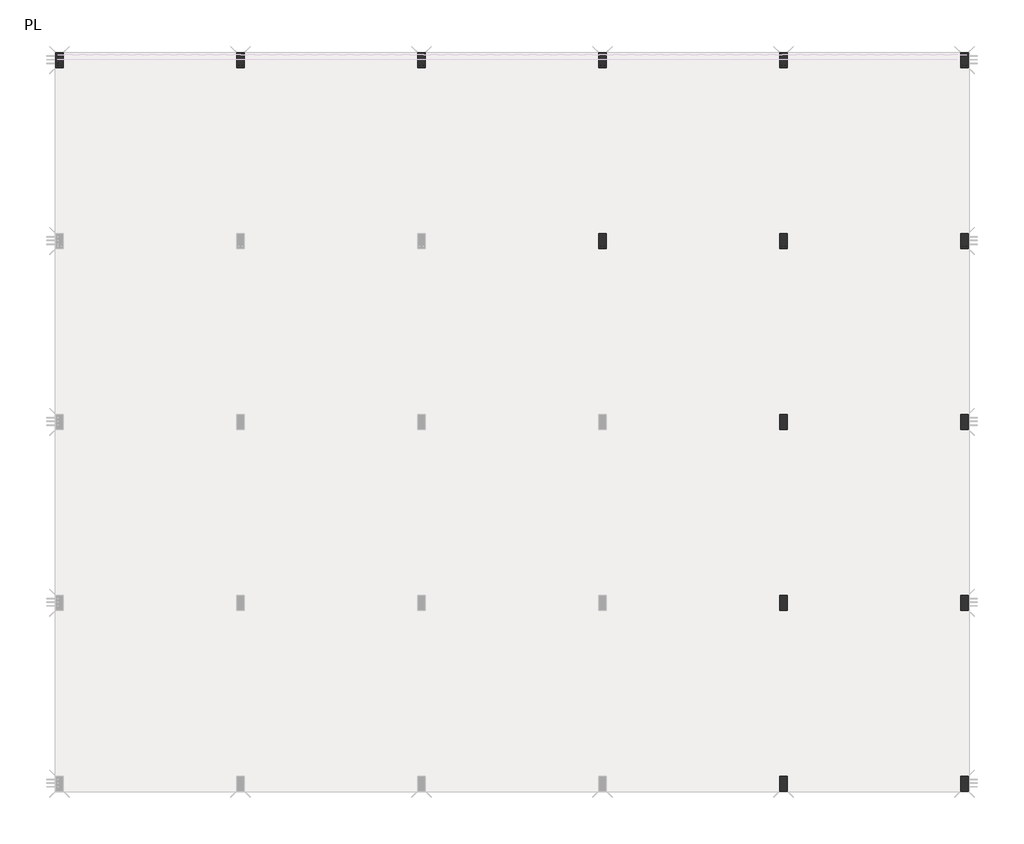
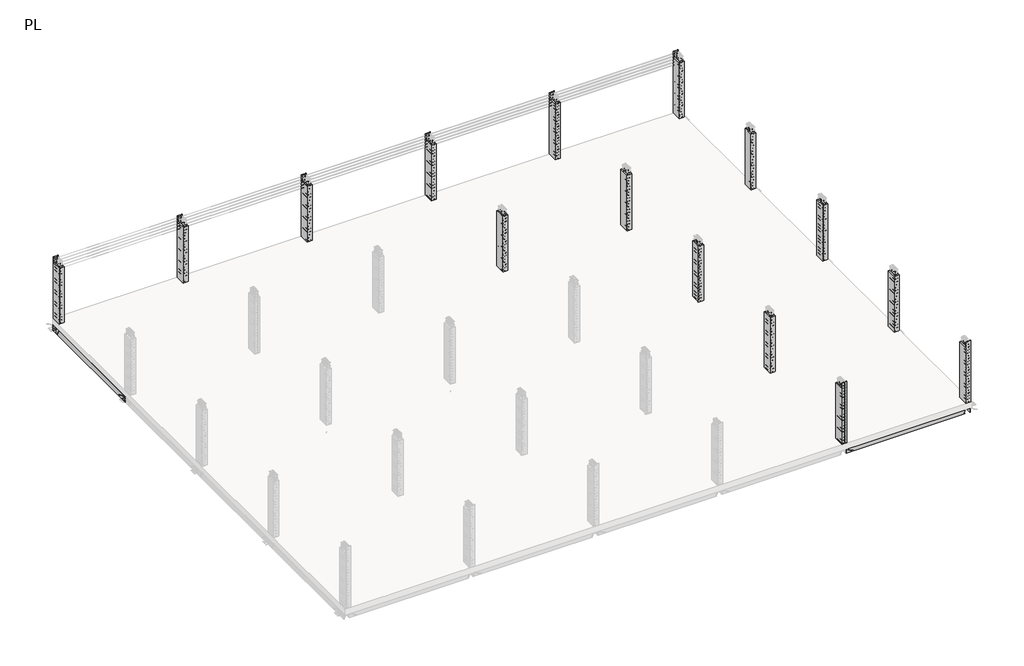
# One storey, part 2 of 10: 25 beams, 15 columns.
"""IFC4 building model written with IfcOpenShell, lengths in millimetres."""

from ifc_helpers import new_model, si_unit, frame, origin, place, context, project, spatial, polyline, outline, extrude, faceted_brep, element, save

model = new_model("IFC4")

# Units and contexts
model_context = context("Model", 3, world=origin())
ifc_project = project(units=[si_unit("LENGTHUNIT", "METRE", prefix="MILLI")], contexts=[model_context])

# Site, building, storey
site = spatial("IfcSite", under=ifc_project)
building = spatial("IfcBuilding", under=site)
storey = spatial("IfcBuildingStorey", under=building, Name="PL", Elevation=271.0)

# Beams
placement = place(None, origin())
element("IfcBeam", 1, ObjectType="Concrete-Rectangular Beam : 300 x 600mm", at=placement, inside=storey, context=model_context, shape_type="Brep", body=[
    faceted_brep([(7798.0455621, 4054.0653602, -329.0), (7823.0455621, 4054.0653602, -329.0), (7823.0455621, 4054.0653602, -29.0), (7798.0455621, 4054.0653602, -29.0), (7823.0455621, 4354.0653602, -329.0), (7798.0455621, 4354.0653602, -329.0), (7798.0455621, 4354.0653602, -29.0), (7823.0455621, 4354.0653602, -29.0)], [[[0, 1, 2, 3]], [[4, 1, 0, 5]], [[4, 5, 6, 7]], [[1, 4, 7, 2]], [[5, 0, 3, 6]], [[3, 2, 7, 6]]]),
    faceted_brep([(-22681.9544379, 4354.0653602, -329.0), (-22681.9544379, 4054.0653602, -329.0), (-22681.9544379, 4054.0653602, -29.0), (-22681.9544379, 4354.0653602, -29.0), (-16835.9544379, 4054.0653602, -329.0), (-16835.9544379, 4354.0653602, -329.0), (-16835.9544379, 4354.0653602, -29.0), (-16835.9544379, 4054.0653602, -29.0), (-22656.9544379, 4054.0653602, -329.0), (-16860.9544379, 4054.0653602, -329.0), (-16860.9544379, 4054.0653602, -29.0), (-22656.9544379, 4054.0653602, -29.0)], [[[0, 1, 2, 3]], [[4, 5, 6, 7]], [[1, 8, 9, 4, 7, 10, 11, 2]], [[1, 0, 5, 4, 9, 8]], [[5, 0, 3, 6]], [[3, 2, 11, 10, 7, 6]]]),
    faceted_brep([(7548.0455621, 4054.0653602, -329.0), (7548.0455621, 4354.0653602, -329.0), (7548.0455621, 4354.0653602, -29.0), (7548.0455621, 4054.0653602, -29.0), (1702.0455621, 4354.0653602, -329.0), (1702.0455621, 4054.0653602, -329.0), (1702.0455621, 4054.0653602, -29.0), (1702.0455621, 4354.0653602, -29.0), (1727.0455621, 4054.0653602, -329.0), (7523.0455621, 4054.0653602, -329.0), (7523.0455621, 4054.0653602, -29.0), (1727.0455621, 4054.0653602, -29.0)], [[[0, 1, 2, 3]], [[4, 5, 6, 7]], [[5, 8, 9, 0, 3, 10, 11, 6]], [[1, 0, 9, 8, 5, 4]], [[1, 4, 7, 2]], [[3, 2, 7, 6, 11, 10]]]),
    faceted_brep([(-16585.9544379, 4354.0653602, -329.0), (-16585.9544379, 4054.0653602, -329.0), (-16585.9544379, 4054.0653602, -29.0), (-16585.9544379, 4354.0653602, -29.0), (-10739.9544379, 4054.0653602, -329.0), (-10739.9544379, 4354.0653602, -329.0), (-10739.9544379, 4354.0653602, -29.0), (-10739.9544379, 4054.0653602, -29.0)], [[[0, 1, 2, 3]], [[4, 5, 6, 7]], [[1, 4, 7, 2]], [[1, 0, 5, 4]], [[5, 0, 3, 6]], [[3, 2, 7, 6]]]),
    faceted_brep([(-10489.9544379, 4354.0653602, -329.0), (-10489.9544379, 4054.0653602, -329.0), (-10489.9544379, 4054.0653602, -29.0), (-10489.9544379, 4354.0653602, -29.0), (-4643.9544379, 4054.0653602, -329.0), (-4643.9544379, 4354.0653602, -329.0), (-4643.9544379, 4354.0653602, -29.0), (-4643.9544379, 4054.0653602, -29.0), (-10464.9544379, 4054.0653602, -329.0), (-10464.9544379, 4054.0653602, -29.0)], [[[0, 1, 2, 3]], [[4, 5, 6, 7]], [[1, 8, 4, 7, 9, 2]], [[1, 0, 5, 4, 8]], [[5, 0, 3, 6]], [[3, 2, 9, 7, 6]]]),
    faceted_brep([(-4393.9544379, 4354.0653602, -329.0), (-4393.9544379, 4054.0653602, -329.0), (-4393.9544379, 4054.0653602, -29.0), (-4393.9544379, 4354.0653602, -29.0), (1452.0455621, 4054.0653602, -329.0), (1452.0455621, 4354.0653602, -329.0), (1452.0455621, 4354.0653602, -29.0), (1452.0455621, 4054.0653602, -29.0), (-4368.9544379, 4054.0653602, -329.0), (-4368.9544379, 4054.0653602, -29.0)], [[[0, 1, 2, 3]], [[4, 5, 6, 7]], [[1, 8, 4, 7, 9, 2]], [[1, 0, 5, 4, 8]], [[5, 0, 3, 6]], [[3, 2, 9, 7, 6]]]),
    faceted_brep([(-22956.9544379, 4354.0653602, -329.0), (-22956.9544379, 4054.0653602, -329.0), (-22956.9544379, 4054.0653602, -29.0), (-22956.9544379, 4354.0653602, -29.0), (-22931.9544379, 4054.0653602, -329.0), (-22931.9544379, 4354.0653602, -329.0), (-22931.9544379, 4354.0653602, -29.0), (-22931.9544379, 4054.0653602, -29.0)], [[[0, 1, 2, 3]], [[4, 5, 6, 7]], [[1, 4, 7, 2]], [[1, 0, 5, 4]], [[5, 0, 3, 6]], [[3, 2, 7, 6]]]),
])
element("IfcBeam", 2, ObjectType="Concrete-Rectangular Beam : 300 x 600mm", at=placement, inside=storey, context=model_context, shape_type="Brep", body=[
    faceted_brep([(7798.0455621, -20429.1167521, -329.0), (7823.0455621, -20429.1167521, -329.0), (7823.0455621, -20429.1167521, -29.0), (7798.0455621, -20429.1167521, -29.0), (7823.0455621, -20129.1167521, -329.0), (7798.0455621, -20129.1167521, -329.0), (7798.0455621, -20129.1167521, -29.0), (7823.0455621, -20129.1167521, -29.0)], [[[0, 1, 2, 3]], [[4, 1, 0, 5]], [[4, 5, 6, 7]], [[1, 4, 7, 2]], [[5, 0, 3, 6]], [[3, 2, 7, 6]]]),
    faceted_brep([(1727.0455621, -20129.1167521, -329.0), (1727.0455621, -20429.1167521, -329.0), (1727.0455621, -20429.1167521, -29.0), (1727.0455621, -20129.1167521, -29.0), (7548.0455621, -20429.1167521, -329.0), (7548.0455621, -20129.1167521, -329.0), (7548.0455621, -20129.1167521, -29.0), (7548.0455621, -20429.1167521, -29.0), (7523.0455621, -20129.1167521, -329.0), (7523.0455621, -20129.1167521, -29.0)], [[[0, 1, 2, 3]], [[4, 5, 6, 7]], [[1, 4, 7, 2]], [[1, 0, 8, 5, 4]], [[5, 8, 0, 3, 9, 6]], [[3, 2, 7, 6, 9]]]),
])
element("IfcBeam", 3, ObjectType="Concrete-Rectangular Beam : 300 x 600mm", at=placement, inside=storey, context=model_context, shape_type="Brep", body=[
    faceted_brep([(7798.0455621, -14333.1167521, -329.0), (7823.0455621, -14333.1167521, -329.0), (7823.0455621, -14333.1167521, -29.0), (7798.0455621, -14333.1167521, -29.0), (7823.0455621, -14033.1167521, -329.0), (7798.0455621, -14033.1167521, -329.0), (7798.0455621, -14033.1167521, -29.0), (7823.0455621, -14033.1167521, -29.0)], [[[0, 1, 2, 3]], [[4, 1, 0, 5]], [[4, 5, 6, 7]], [[1, 4, 7, 2]], [[5, 0, 3, 6]], [[3, 2, 7, 6]]]),
    faceted_brep([(1727.0455621, -14033.1167521, -329.0), (1727.0455621, -14333.1167521, -329.0), (1727.0455621, -14333.1167521, -29.0), (1727.0455621, -14033.1167521, -29.0), (7548.0455621, -14333.1167521, -329.0), (7548.0455621, -14033.1167521, -329.0), (7548.0455621, -14033.1167521, -29.0), (7548.0455621, -14333.1167521, -29.0), (7523.0455621, -14333.1167521, -329.0), (7523.0455621, -14333.1167521, -29.0), (7523.0455621, -14033.1167521, -329.0), (7523.0455621, -14033.1167521, -29.0)], [[[0, 1, 2, 3]], [[4, 5, 6, 7]], [[1, 8, 4, 7, 9, 2]], [[1, 0, 10, 5, 4, 8]], [[5, 10, 0, 3, 11, 6]], [[3, 2, 9, 7, 6, 11]]]),
])
element("IfcBeam", 4, ObjectType="Concrete-Rectangular Beam : 300 x 600mm", at=placement, inside=storey, context=model_context, shape_type="Brep", body=[
    faceted_brep([(7798.0455621, -8237.1167521, -329.0), (7823.0455621, -8237.1167521, -329.0), (7823.0455621, -8237.1167521, -29.0), (7798.0455621, -8237.1167521, -29.0), (7823.0455621, -7937.1167521, -329.0), (7798.0455621, -7937.1167521, -329.0), (7798.0455621, -7937.1167521, -29.0), (7823.0455621, -7937.1167521, -29.0)], [[[0, 1, 2, 3]], [[4, 1, 0, 5]], [[4, 5, 6, 7]], [[1, 4, 7, 2]], [[5, 0, 3, 6]], [[3, 2, 7, 6]]]),
    faceted_brep([(1727.0455621, -7937.1167521, -329.0), (1727.0455621, -8237.1167521, -329.0), (1727.0455621, -8237.1167521, -29.0), (1727.0455621, -7937.1167521, -29.0), (7548.0455621, -8237.1167521, -329.0), (7548.0455621, -7937.1167521, -329.0), (7548.0455621, -7937.1167521, -29.0), (7548.0455621, -8237.1167521, -29.0), (7523.0455621, -8237.1167521, -329.0), (7523.0455621, -8237.1167521, -29.0), (7523.0455621, -7937.1167521, -329.0), (7523.0455621, -7937.1167521, -29.0)], [[[0, 1, 2, 3]], [[4, 5, 6, 7]], [[1, 8, 4, 7, 9, 2]], [[1, 0, 10, 5, 4, 8]], [[5, 10, 0, 3, 11, 6]], [[3, 2, 9, 7, 6, 11]]]),
])
element("IfcBeam", 5, ObjectType="Concrete-Rectangular Beam : 300 x 600mm", at=placement, inside=storey, context=model_context, shape_type="Brep", body=[
    faceted_brep([(-4393.9544379, -2141.1167521, -329.0), (-4368.9544379, -2141.1167521, -329.0), (-4368.9544379, -2141.1167521, -29.0), (-4393.9544379, -2141.1167521, -29.0), (-4368.9544379, -1841.1167521, -329.0), (-4393.9544379, -1841.1167521, -329.0), (-4393.9544379, -1841.1167521, -29.0), (-4368.9544379, -1841.1167521, -29.0)], [[[0, 1, 2, 3]], [[4, 1, 0, 5]], [[4, 5, 6, 7]], [[1, 4, 7, 2]], [[5, 0, 3, 6]], [[3, 2, 7, 6]]]),
    faceted_brep([(-10464.9544379, -1841.1167521, -329.0), (-10464.9544379, -2141.1167521, -329.0), (-10464.9544379, -2141.1167521, -29.0), (-10464.9544379, -1841.1167521, -29.0), (-4643.9544379, -2141.1167521, -329.0), (-4643.9544379, -1841.1167521, -329.0), (-4643.9544379, -1841.1167521, -29.0), (-4643.9544379, -2141.1167521, -29.0), (-4668.9544379, -2141.1167521, -329.0), (-4668.9544379, -2141.1167521, -29.0), (-4668.9544379, -1841.1167521, -329.0), (-4668.9544379, -1841.1167521, -29.0)], [[[0, 1, 2, 3]], [[4, 5, 6, 7]], [[1, 8, 4, 7, 9, 2]], [[1, 0, 10, 5, 4, 8]], [[5, 10, 0, 3, 11, 6]], [[3, 2, 9, 7, 6, 11]]]),
])
element("IfcBeam", 6, ObjectType="Concrete-Rectangular Beam : 300 x 600mm", at=placement, inside=storey, context=model_context, shape_type="Brep", body=[
    faceted_brep([(1702.0455621, -2141.1167521, -329.0), (1727.0455621, -2141.1167521, -329.0), (1727.0455621, -2141.1167521, -29.0), (1702.0455621, -2141.1167521, -29.0), (1727.0455621, -1841.1167521, -329.0), (1702.0455621, -1841.1167521, -329.0), (1702.0455621, -1841.1167521, -29.0), (1727.0455621, -1841.1167521, -29.0)], [[[0, 1, 2, 3]], [[4, 1, 0, 5]], [[4, 5, 6, 7]], [[1, 4, 7, 2]], [[5, 0, 3, 6]], [[3, 2, 7, 6]]]),
    faceted_brep([(-4368.9544379, -1841.1167521, -329.0), (-4368.9544379, -2141.1167521, -329.0), (-4368.9544379, -2141.1167521, -29.0), (-4368.9544379, -1841.1167521, -29.0), (1452.0455621, -2141.1167521, -329.0), (1452.0455621, -1841.1167521, -329.0), (1452.0455621, -1841.1167521, -29.0), (1452.0455621, -2141.1167521, -29.0), (1427.0455621, -2141.1167521, -329.0), (1427.0455621, -2141.1167521, -29.0), (1427.0455621, -1841.1167521, -329.0), (1427.0455621, -1841.1167521, -29.0)], [[[0, 1, 2, 3]], [[4, 5, 6, 7]], [[1, 8, 4, 7, 9, 2]], [[1, 0, 10, 5, 4, 8]], [[5, 10, 0, 3, 11, 6]], [[3, 2, 9, 7, 6, 11]]]),
])
element("IfcBeam", 7, ObjectType="Concrete-Rectangular Beam : 300 x 600mm", at=placement, inside=storey, context=model_context, shape_type="Brep", body=[
    faceted_brep([(7798.0455621, -2141.1167521, -329.0), (7823.0455621, -2141.1167521, -329.0), (7823.0455621, -2141.1167521, -29.0), (7798.0455621, -2141.1167521, -29.0), (7823.0455621, -1841.1167521, -329.0), (7798.0455621, -1841.1167521, -329.0), (7798.0455621, -1841.1167521, -29.0), (7823.0455621, -1841.1167521, -29.0)], [[[0, 1, 2, 3]], [[4, 1, 0, 5]], [[4, 5, 6, 7]], [[1, 4, 7, 2]], [[5, 0, 3, 6]], [[3, 2, 7, 6]]]),
    faceted_brep([(1727.0455621, -1841.1167521, -329.0), (1727.0455621, -2141.1167521, -329.0), (1727.0455621, -2141.1167521, -29.0), (1727.0455621, -1841.1167521, -29.0), (7548.0455621, -2141.1167521, -329.0), (7548.0455621, -1841.1167521, -329.0), (7548.0455621, -1841.1167521, -29.0), (7548.0455621, -2141.1167521, -29.0), (7523.0455621, -2141.1167521, -329.0), (7523.0455621, -2141.1167521, -29.0), (7523.0455621, -1841.1167521, -329.0), (7523.0455621, -1841.1167521, -29.0)], [[[0, 1, 2, 3]], [[4, 5, 6, 7]], [[1, 8, 4, 7, 9, 2]], [[1, 0, 10, 5, 4, 8]], [[5, 10, 0, 3, 11, 6]], [[3, 2, 9, 7, 6, 11]]]),
])
element("IfcBeam", 8, ObjectType="Concrete-Rectangular Beam : 300 x 600mm", at=placement, inside=storey, context=model_context, shape_type="Brep", body=[
    faceted_brep([(-10489.9544379, 3954.8832479, -329.0), (-10464.9544379, 3954.8832479, -329.0), (-10464.9544379, 3954.8832479, -29.0), (-10489.9544379, 3954.8832479, -29.0), (-10464.9544379, 4054.0653602, -329.0), (-10489.9544379, 4054.0653602, -329.0), (-10464.9544379, 4054.0653602, -29.0), (-10489.9544379, 4054.0653602, -29.0)], [[[0, 1, 2, 3]], [[4, 1, 0, 5]], [[1, 4, 6, 2]], [[5, 0, 3, 7]], [[4, 5, 7, 6]], [[3, 2, 6, 7]]]),
    faceted_brep([(-16860.9544379, 4054.0653602, -329.0), (-16860.9544379, 3954.8832479, -329.0), (-16860.9544379, 3954.8832479, -29.0), (-16860.9544379, 4054.0653602, -29.0), (-16835.9544379, 3954.8832479, -329.0), (-16835.9544379, 4054.0653602, -329.0), (-16835.9544379, 4054.0653602, -29.0), (-16835.9544379, 3954.8832479, -29.0)], [[[0, 1, 2, 3]], [[4, 5, 6, 7]], [[1, 4, 7, 2]], [[1, 0, 5, 4]], [[5, 0, 3, 6]], [[3, 2, 7, 6]]]),
    faceted_brep([(-10739.9544379, 3954.8832479, -329.0), (-10739.9544379, 4054.0653602, -329.0), (-10739.9544379, 4054.0653602, -29.0), (-10739.9544379, 3954.8832479, -29.0), (-16585.9544379, 3954.8832479, -329.0), (-16560.9544379, 3954.8832479, -329.0), (-10764.9544379, 3954.8832479, -329.0), (-10764.9544379, 3954.8832479, -29.0), (-16560.9544379, 3954.8832479, -29.0), (-16585.9544379, 3954.8832479, -29.0), (-16585.9544379, 4054.0653602, -329.0), (-16585.9544379, 4054.0653602, -29.0)], [[[0, 1, 2, 3]], [[4, 5, 6, 0, 3, 7, 8, 9]], [[1, 0, 6, 5, 4, 10]], [[1, 10, 11, 2]], [[10, 4, 9, 11]], [[3, 2, 11, 9, 8, 7]]]),
])
element("IfcBeam", 9, ObjectType="Concrete-Rectangular Beam : 300 x 600mm", at=placement, inside=storey, context=model_context, shape_type="Brep", body=[
    faceted_brep([(-4393.9544379, 3954.8832479, -329.0), (-4368.9544379, 3954.8832479, -329.0), (-4368.9544379, 3954.8832479, -29.0), (-4393.9544379, 3954.8832479, -29.0), (-4393.9544379, 4054.0653602, -329.0), (-4368.9544379, 4054.0653602, -329.0), (-4368.9544379, 4054.0653602, -29.0), (-4393.9544379, 4054.0653602, -29.0)], [[[0, 1, 2, 3]], [[1, 0, 4, 5]], [[1, 5, 6, 2]], [[4, 0, 3, 7]], [[5, 4, 7, 6]], [[3, 2, 6, 7]]]),
    faceted_brep([(-10464.9544379, 4054.0653602, -329.0), (-10464.9544379, 3954.8832479, -329.0), (-10464.9544379, 3954.8832479, -29.0), (-10464.9544379, 4054.0653602, -29.0), (-4643.9544379, 3954.8832479, -329.0), (-4643.9544379, 4054.0653602, -329.0), (-4643.9544379, 4054.0653602, -29.0), (-4643.9544379, 3954.8832479, -29.0), (-4668.9544379, 3954.8832479, -329.0), (-4668.9544379, 3954.8832479, -29.0)], [[[0, 1, 2, 3]], [[4, 5, 6, 7]], [[1, 8, 4, 7, 9, 2]], [[4, 8, 1, 0, 5]], [[5, 0, 3, 6]], [[3, 2, 9, 7, 6]]]),
])
element("IfcBeam", 10, ObjectType="Concrete-Rectangular Beam : 300 x 600mm", at=placement, inside=storey, context=model_context, shape_type="Brep", body=[
    faceted_brep([(1702.0455621, 3954.8832479, -329.0), (1727.0455621, 3954.8832479, -329.0), (1727.0455621, 3954.8832479, -29.0), (1702.0455621, 3954.8832479, -29.0), (1702.0455621, 4054.0653602, -329.0), (1727.0455621, 4054.0653602, -329.0), (1727.0455621, 4054.0653602, -29.0), (1702.0455621, 4054.0653602, -29.0)], [[[0, 1, 2, 3]], [[1, 0, 4, 5]], [[1, 5, 6, 2]], [[4, 0, 3, 7]], [[5, 4, 7, 6]], [[3, 2, 6, 7]]]),
    faceted_brep([(-4368.9544379, 4054.0653602, -329.0), (-4368.9544379, 3954.8832479, -329.0), (-4368.9544379, 3954.8832479, -29.0), (-4368.9544379, 4054.0653602, -29.0), (1452.0455621, 3954.8832479, -329.0), (1452.0455621, 4054.0653602, -329.0), (1452.0455621, 4054.0653602, -29.0), (1452.0455621, 3954.8832479, -29.0), (1427.0455621, 3954.8832479, -329.0), (1427.0455621, 3954.8832479, -29.0)], [[[0, 1, 2, 3]], [[4, 5, 6, 7]], [[1, 8, 4, 7, 9, 2]], [[4, 8, 1, 0, 5]], [[5, 0, 3, 6]], [[3, 2, 9, 7, 6]]]),
])
element("IfcBeam", 11, ObjectType="Concrete-Rectangular Beam : 300 x 600mm", at=placement, inside=storey, context=model_context, shape_type="SweptSolid", body=[
    extrude(outline(polyline([(1727.0455621, 3954.8832479), (1727.0455621, 4054.0653602), (7523.0455621, 4054.0653602), (7523.0455621, 3954.8832479), (1727.0455621, 3954.8832479)])), frame((0.0, 0.0, -329.0), z_axis=(0.0, 0.0, 1.0), x_axis=(1.0, 0.0, 0.0)), (0.0, 0.0, 1.0), 300.0),
])
element("IfcBeam", 12, ObjectType="Concrete-Rectangular Beam : 300 x 600mm", at=placement, inside=storey, context=model_context, shape_type="Brep", body=[
    faceted_brep([(-22656.9544379, -1841.1167521, -329.0), (-22656.9544379, 3954.8832479, -329.0), (-22656.9544379, 4054.0653602, -329.0), (-22656.9544379, 4054.0653602, -29.0), (-22656.9544379, 3954.8832479, -29.0), (-22656.9544379, -1841.1167521, -29.0), (-22956.9544379, 4054.0653602, -329.0), (-22931.9544379, 4054.0653602, -329.0), (-22931.9544379, 3854.8832479, -329.0), (-22681.9544379, 3854.8832479, -329.0), (-22681.9544379, 4054.0653602, -329.0), (-22681.9544379, -1841.1167521, -329.0), (-22681.9544379, -1741.1167521, -329.0), (-22931.9544379, -1741.1167521, -329.0), (-22931.9544379, -1841.1167521, -329.0), (-22956.9544379, -1841.1167521, -329.0), (-22956.9544379, -1841.1167521, -29.0), (-22956.9544379, 4054.0653602, -29.0), (-22681.9544379, 4054.0653602, -29.0), (-22931.9544379, 4054.0653602, -29.0), (-22931.9544379, 3854.8832479, -29.0), (-22681.9544379, 3854.8832479, -29.0), (-22681.9544379, -1741.1167521, -29.0), (-22931.9544379, -1741.1167521, -29.0), (-22931.9544379, -1841.1167521, -29.0), (-22681.9544379, -1841.1167521, -29.0)], [[[0, 1, 2, 3, 4, 5]], [[6, 7, 8, 9, 10, 2, 1, 0, 11, 12, 13, 14, 15]], [[6, 15, 16, 17]], [[2, 10, 18, 3]], [[8, 7, 19, 20]], [[9, 8, 20, 21]], [[10, 9, 21, 18]], [[7, 6, 17, 19]], [[13, 12, 22, 23]], [[14, 13, 23, 24]], [[12, 11, 25, 22]], [[11, 0, 5, 25]], [[15, 14, 24, 16]], [[5, 4, 3, 18, 21, 20, 19, 17, 16, 24, 23, 22, 25]]]),
])
element("IfcBeam", 13, ObjectType="Concrete-Rectangular Beam : 300 x 600mm", at=placement, inside=storey, context=model_context, shape_type="SweptSolid", body=[
    extrude(outline(polyline([(-16585.9544379, -1741.1167521), (-16835.9544379, -1741.1167521), (-16835.9544379, -1841.1167521), (-16860.9544379, -1841.1167521), (-16860.9544379, 3954.8832479), (-16835.9544379, 3954.8832479), (-16835.9544379, 3854.8832479), (-16585.9544379, 3854.8832479), (-16585.9544379, 3954.8832479), (-16560.9544379, 3954.8832479), (-16560.9544379, -1841.1167521), (-16585.9544379, -1841.1167521), (-16585.9544379, -1741.1167521)])), frame((0.0, 0.0, -329.0), z_axis=(0.0, 0.0, 1.0), x_axis=(1.0, 0.0, 0.0)), (0.0, 0.0, 1.0), 300.0),
])
element("IfcBeam", 14, ObjectType="Concrete-Rectangular Beam : 300 x 600mm", at=placement, inside=storey, context=model_context, shape_type="SweptSolid", body=[
    extrude(outline(polyline([(-10489.9544379, -1741.1167521), (-10739.9544379, -1741.1167521), (-10739.9544379, -1841.1167521), (-10764.9544379, -1841.1167521), (-10764.9544379, 3954.8832479), (-10739.9544379, 3954.8832479), (-10739.9544379, 3854.8832479), (-10489.9544379, 3854.8832479), (-10489.9544379, 3954.8832479), (-10464.9544379, 3954.8832479), (-10464.9544379, -1841.1167521), (-10489.9544379, -1841.1167521), (-10489.9544379, -1741.1167521)])), frame((0.0, 0.0, -329.0), z_axis=(0.0, 0.0, 1.0), x_axis=(1.0, 0.0, 0.0)), (0.0, 0.0, 1.0), 300.0),
])
element("IfcBeam", 15, ObjectType="Concrete-Rectangular Beam : 300 x 600mm", at=placement, inside=storey, context=model_context, shape_type="SweptSolid", body=[
    extrude(outline(polyline([(-4643.9544379, -7937.1167521), (-4668.9544379, -7937.1167521), (-4668.9544379, -2141.1167521), (-4643.9544379, -2141.1167521), (-4643.9544379, -2241.1167521), (-4393.9544379, -2241.1167521), (-4393.9544379, -2141.1167521), (-4368.9544379, -2141.1167521), (-4368.9544379, -7937.1167521), (-4393.9544379, -7937.1167521), (-4393.9544379, -7837.1167521), (-4643.9544379, -7837.1167521), (-4643.9544379, -7937.1167521)])), frame((0.0, 0.0, -329.0), z_axis=(0.0, 0.0, 1.0), x_axis=(1.0, 0.0, 0.0)), (0.0, 0.0, 1.0), 300.0),
])
element("IfcBeam", 16, ObjectType="Concrete-Rectangular Beam : 300 x 600mm", at=placement, inside=storey, context=model_context, shape_type="SweptSolid", body=[
    extrude(outline(polyline([(-4393.9544379, -1741.1167521), (-4643.9544379, -1741.1167521), (-4643.9544379, -1841.1167521), (-4668.9544379, -1841.1167521), (-4668.9544379, 3954.8832479), (-4643.9544379, 3954.8832479), (-4643.9544379, 3854.8832479), (-4393.9544379, 3854.8832479), (-4393.9544379, 3954.8832479), (-4368.9544379, 3954.8832479), (-4368.9544379, -1841.1167521), (-4393.9544379, -1841.1167521), (-4393.9544379, -1741.1167521)])), frame((0.0, 0.0, -329.0), z_axis=(0.0, 0.0, 1.0), x_axis=(1.0, 0.0, 0.0)), (0.0, 0.0, 1.0), 300.0),
])
element("IfcBeam", 17, ObjectType="Concrete-Rectangular Beam : 300 x 600mm", at=placement, inside=storey, context=model_context, shape_type="SweptSolid", body=[
    extrude(outline(polyline([(1452.0455621, -20129.1167521), (1427.0455621, -20129.1167521), (1427.0455621, -14333.1167521), (1452.0455621, -14333.1167521), (1452.0455621, -14433.1167521), (1702.0455621, -14433.1167521), (1702.0455621, -14333.1167521), (1727.0455621, -14333.1167521), (1727.0455621, -20129.1167521), (1702.0455621, -20129.1167521), (1702.0455621, -20029.1167521), (1452.0455621, -20029.1167521), (1452.0455621, -20129.1167521)])), frame((0.0, 0.0, -329.0), z_axis=(0.0, 0.0, 1.0), x_axis=(1.0, 0.0, 0.0)), (0.0, 0.0, 1.0), 300.0),
])
element("IfcBeam", 18, ObjectType="Concrete-Rectangular Beam : 300 x 600mm", at=placement, inside=storey, context=model_context, shape_type="SweptSolid", body=[
    extrude(outline(polyline([(1452.0455621, -14033.1167521), (1427.0455621, -14033.1167521), (1427.0455621, -8237.1167521), (1452.0455621, -8237.1167521), (1452.0455621, -8337.1167521), (1702.0455621, -8337.1167521), (1702.0455621, -8237.1167521), (1727.0455621, -8237.1167521), (1727.0455621, -14033.1167521), (1702.0455621, -14033.1167521), (1702.0455621, -13933.1167521), (1452.0455621, -13933.1167521), (1452.0455621, -14033.1167521)])), frame((0.0, 0.0, -329.0), z_axis=(0.0, 0.0, 1.0), x_axis=(1.0, 0.0, 0.0)), (0.0, 0.0, 1.0), 300.0),
])
element("IfcBeam", 19, ObjectType="Concrete-Rectangular Beam : 300 x 600mm", at=placement, inside=storey, context=model_context, shape_type="SweptSolid", body=[
    extrude(outline(polyline([(1452.0455621, -7937.1167521), (1427.0455621, -7937.1167521), (1427.0455621, -2141.1167521), (1452.0455621, -2141.1167521), (1452.0455621, -2241.1167521), (1702.0455621, -2241.1167521), (1702.0455621, -2141.1167521), (1727.0455621, -2141.1167521), (1727.0455621, -7937.1167521), (1702.0455621, -7937.1167521), (1702.0455621, -7837.1167521), (1452.0455621, -7837.1167521), (1452.0455621, -7937.1167521)])), frame((0.0, 0.0, -329.0), z_axis=(0.0, 0.0, 1.0), x_axis=(1.0, 0.0, 0.0)), (0.0, 0.0, 1.0), 300.0),
])
element("IfcBeam", 20, ObjectType="Concrete-Rectangular Beam : 300 x 600mm", at=placement, inside=storey, context=model_context, shape_type="SweptSolid", body=[
    extrude(outline(polyline([(1452.0455621, -1841.1167521), (1427.0455621, -1841.1167521), (1427.0455621, 3954.8832479), (1452.0455621, 3954.8832479), (1452.0455621, 3854.8832479), (1702.0455621, 3854.8832479), (1702.0455621, 3954.8832479), (1727.0455621, 3954.8832479), (1727.0455621, -1841.1167521), (1702.0455621, -1841.1167521), (1702.0455621, -1741.1167521), (1452.0455621, -1741.1167521), (1452.0455621, -1841.1167521)])), frame((0.0, 0.0, -329.0), z_axis=(0.0, 0.0, 1.0), x_axis=(1.0, 0.0, 0.0)), (0.0, 0.0, 1.0), 300.0),
])
element("IfcBeam", 21, ObjectType="Concrete-Rectangular Beam : 300 x 600mm", at=placement, inside=storey, context=model_context, shape_type="SweptSolid", body=[
    extrude(outline(polyline([(7548.0455621, -20129.1167521), (7523.0455621, -20129.1167521), (7523.0455621, -14333.1167521), (7548.0455621, -14333.1167521), (7548.0455621, -14433.1167521), (7798.0455621, -14433.1167521), (7798.0455621, -14333.1167521), (7823.0455621, -14333.1167521), (7823.0455621, -20129.1167521), (7798.0455621, -20129.1167521), (7798.0455621, -20029.1167521), (7548.0455621, -20029.1167521), (7548.0455621, -20129.1167521)])), frame((0.0, 0.0, -329.0), z_axis=(0.0, 0.0, 1.0), x_axis=(1.0, 0.0, 0.0)), (0.0, 0.0, 1.0), 300.0),
])
element("IfcBeam", 22, ObjectType="Concrete-Rectangular Beam : 300 x 600mm", at=placement, inside=storey, context=model_context, shape_type="SweptSolid", body=[
    extrude(outline(polyline([(7548.0455621, -14033.1167521), (7523.0455621, -14033.1167521), (7523.0455621, -8237.1167521), (7548.0455621, -8237.1167521), (7548.0455621, -8337.1167521), (7798.0455621, -8337.1167521), (7798.0455621, -8237.1167521), (7823.0455621, -8237.1167521), (7823.0455621, -14033.1167521), (7798.0455621, -14033.1167521), (7798.0455621, -13933.1167521), (7548.0455621, -13933.1167521), (7548.0455621, -14033.1167521)])), frame((0.0, 0.0, -329.0), z_axis=(0.0, 0.0, 1.0), x_axis=(1.0, 0.0, 0.0)), (0.0, 0.0, 1.0), 300.0),
])
element("IfcBeam", 23, ObjectType="Concrete-Rectangular Beam : 300 x 600mm", at=placement, inside=storey, context=model_context, shape_type="SweptSolid", body=[
    extrude(outline(polyline([(7798.0455621, -7837.1167521), (7548.0455621, -7837.1167521), (7548.0455621, -7937.1167521), (7523.0455621, -7937.1167521), (7523.0455621, -2141.1167521), (7548.0455621, -2141.1167521), (7548.0455621, -2241.1167521), (7798.0455621, -2241.1167521), (7798.0455621, -2141.1167521), (7823.0455621, -2141.1167521), (7823.0455621, -7937.1167521), (7798.0455621, -7937.1167521), (7798.0455621, -7837.1167521)])), frame((0.0, 0.0, -329.0), z_axis=(0.0, 0.0, 1.0), x_axis=(1.0, 0.0, 0.0)), (0.0, 0.0, 1.0), 300.0),
])
element("IfcBeam", 24, ObjectType="Concrete-Rectangular Beam : 300 x 600mm", at=placement, inside=storey, context=model_context, shape_type="Brep", body=[
    faceted_brep([(7823.0455621, -1841.1167521, -329.0), (7823.0455621, 4054.0653602, -329.0), (7823.0455621, 4054.0653602, -29.0), (7823.0455621, -1841.1167521, -29.0), (7798.0455621, -1741.1167521, -329.0), (7548.0455621, -1741.1167521, -329.0), (7548.0455621, -1841.1167521, -329.0), (7523.0455621, -1841.1167521, -329.0), (7523.0455621, 3954.8832479, -329.0), (7523.0455621, 4054.0653602, -329.0), (7548.0455621, 4054.0653602, -329.0), (7548.0455621, 3854.8832479, -329.0), (7798.0455621, 3854.8832479, -329.0), (7798.0455621, 4054.0653602, -329.0), (7798.0455621, -1841.1167521, -329.0), (7523.0455621, -1841.1167521, -29.0), (7523.0455621, 3954.8832479, -29.0), (7523.0455621, 4054.0653602, -29.0), (7798.0455621, -1741.1167521, -29.0), (7548.0455621, -1741.1167521, -29.0), (7548.0455621, -1841.1167521, -29.0), (7798.0455621, -1841.1167521, -29.0), (7798.0455621, 4054.0653602, -29.0), (7548.0455621, 4054.0653602, -29.0), (7548.0455621, 3854.8832479, -29.0), (7798.0455621, 3854.8832479, -29.0)], [[[0, 1, 2, 3]], [[4, 5, 6, 7, 8, 9, 10, 11, 12, 13, 1, 0, 14]], [[9, 8, 7, 15, 16, 17]], [[5, 4, 18, 19]], [[6, 5, 19, 20]], [[4, 14, 21, 18]], [[7, 6, 20, 15]], [[14, 0, 3, 21]], [[1, 13, 22, 2]], [[11, 10, 23, 24]], [[12, 11, 24, 25]], [[13, 12, 25, 22]], [[10, 9, 17, 23]], [[3, 2, 22, 25, 24, 23, 17, 16, 15, 20, 19, 18, 21]]]),
])
element("IfcBeam", 25, ObjectType="Concrete-Rectangular Beam : 300 x 600mm", at=placement, inside=storey, context=model_context, shape_type="SweptSolid", body=[
    extrude(outline(polyline([(-22656.9544379, 3954.8832479), (-22656.9544379, 4054.0653602), (-16860.9544379, 4054.0653602), (-16860.9544379, 3954.8832479), (-22656.9544379, 3954.8832479)])), frame((0.0, 0.0, -329.0), z_axis=(0.0, 0.0, 1.0), x_axis=(1.0, 0.0, 0.0)), (0.0, 0.0, 1.0), 300.0),
])

# Columns
element("IfcColumn", 26, ObjectType="Concrete-Rectangular-Column : 500X250", at=placement, inside=storey, context=model_context, shape_type="SweptSolid", body=[
    extrude(outline(polyline([(4354.8832479, 3471.4), (4354.8832479, 265.0), (4354.0653602, 265.0), (4354.0653602, 271.0), (3854.8832479, 271.0), (3854.8832479, 3171.4), (4354.0653602, 3171.4), (4354.0653602, 3471.4), (4354.8832479, 3471.4)])), frame((-22931.9544379, 0.0, 0.0), z_axis=(1.0, 0.0, 0.0), x_axis=(0.0, 1.0, 0.0)), (0.0, 0.0, 1.0), 250.0),
])
element("IfcColumn", 27, ObjectType="Concrete-Rectangular-Column : 500X250", at=placement, inside=storey, context=model_context, shape_type="SweptSolid", body=[
    extrude(outline(polyline([(-20529.1167521, 271.0), (-20529.1167521, 3471.4), (-20525.9346398, 3471.4), (-20525.9346398, 3171.4), (-20029.1167521, 3171.4), (-20029.1167521, 271.0), (-20529.1167521, 271.0)])), frame((1452.0455621, 0.0, 0.0), z_axis=(1.0, 0.0, 0.0), x_axis=(0.0, 1.0, 0.0)), (0.0, 0.0, 1.0), 250.0),
])
element("IfcColumn", 28, ObjectType="Concrete-Rectangular-Column : 500X250", at=placement, inside=storey, context=model_context, shape_type="SweptSolid", body=[
    extrude(outline(polyline([(-20529.1167521, 271.0), (-20529.1167521, 3471.4), (-20525.9346398, 3471.4), (-20525.9346398, 3171.4), (-20029.1167521, 3171.4), (-20029.1167521, 271.0), (-20529.1167521, 271.0)])), frame((7548.0455621, 0.0, 0.0), z_axis=(1.0, 0.0, 0.0), x_axis=(0.0, 1.0, 0.0)), (0.0, 0.0, 1.0), 250.0),
])
element("IfcColumn", 29, ObjectType="Concrete-Rectangular-Column : 500X250", at=placement, inside=storey, context=model_context, shape_type="SweptSolid", body=[
    extrude(outline(polyline([(1452.0455621, -13933.1167521), (1702.0455621, -13933.1167521), (1702.0455621, -14433.1167521), (1452.0455621, -14433.1167521), (1452.0455621, -13933.1167521)])), frame((0.0, 0.0, 271.0), z_axis=(0.0, 0.0, 1.0), x_axis=(1.0, 0.0, 0.0)), (0.0, 0.0, 1.0), 2900.4),
])
element("IfcColumn", 30, ObjectType="Concrete-Rectangular-Column : 500X250", at=placement, inside=storey, context=model_context, shape_type="SweptSolid", body=[
    extrude(outline(polyline([(7548.0455621, -13933.1167521), (7798.0455621, -13933.1167521), (7798.0455621, -14433.1167521), (7548.0455621, -14433.1167521), (7548.0455621, -13933.1167521)])), frame((0.0, 0.0, 271.0), z_axis=(0.0, 0.0, 1.0), x_axis=(1.0, 0.0, 0.0)), (0.0, 0.0, 1.0), 2900.4),
])
element("IfcColumn", 31, ObjectType="Concrete-Rectangular-Column : 500X250", at=placement, inside=storey, context=model_context, shape_type="SweptSolid", body=[
    extrude(outline(polyline([(1452.0455621, -7837.1167521), (1702.0455621, -7837.1167521), (1702.0455621, -8337.1167521), (1452.0455621, -8337.1167521), (1452.0455621, -7837.1167521)])), frame((0.0, 0.0, 271.0), z_axis=(0.0, 0.0, 1.0), x_axis=(1.0, 0.0, 0.0)), (0.0, 0.0, 1.0), 2900.4),
])
element("IfcColumn", 32, ObjectType="Concrete-Rectangular-Column : 500X250", at=placement, inside=storey, context=model_context, shape_type="SweptSolid", body=[
    extrude(outline(polyline([(7548.0455621, -7837.1167521), (7798.0455621, -7837.1167521), (7798.0455621, -8337.1167521), (7548.0455621, -8337.1167521), (7548.0455621, -7837.1167521)])), frame((0.0, 0.0, 271.0), z_axis=(0.0, 0.0, 1.0), x_axis=(1.0, 0.0, 0.0)), (0.0, 0.0, 1.0), 2900.4),
])
element("IfcColumn", 33, ObjectType="Concrete-Rectangular-Column : 500X250", at=placement, inside=storey, context=model_context, shape_type="Brep", body=[
    faceted_brep([(-4393.9544379, -1741.1167521, 271.0), (-4643.9544379, -1741.1167521, 271.0), (-4643.9544379, -1741.1167521, 3171.4), (-4393.9544379, -1741.1167521, 3171.4), (-4643.9544379, -2241.1167521, 271.0), (-4643.9544379, -2241.1167521, 3171.4), (-4643.9544379, -2141.1167521, 3171.4), (-4643.9544379, -1841.1167521, 3171.4), (-4393.9544379, -2241.1167521, 271.0), (-4393.9544379, -2241.1167521, 3171.4), (-4393.9544379, -1841.1167521, 3171.4), (-4393.9544379, -2141.1167521, 3171.4)], [[[0, 1, 2, 3]], [[1, 4, 5, 6, 7, 2]], [[4, 8, 9, 5]], [[8, 0, 3, 10, 11, 9]], [[1, 0, 8, 4]], [[3, 2, 7, 6, 5, 9, 11, 10]]]),
])
element("IfcColumn", 34, ObjectType="Concrete-Rectangular-Column : 500X250", at=placement, inside=storey, context=model_context, shape_type="Brep", body=[
    faceted_brep([(1702.0455621, -1741.1167521, 271.0), (1452.0455621, -1741.1167521, 271.0), (1452.0455621, -1741.1167521, 3171.4), (1702.0455621, -1741.1167521, 3171.4), (1452.0455621, -2241.1167521, 271.0), (1452.0455621, -2241.1167521, 3171.4), (1452.0455621, -2141.1167521, 3171.4), (1452.0455621, -1841.1167521, 3171.4), (1702.0455621, -2241.1167521, 271.0), (1702.0455621, -2241.1167521, 3171.4), (1702.0455621, -1841.1167521, 3171.4), (1702.0455621, -2141.1167521, 3171.4)], [[[0, 1, 2, 3]], [[1, 4, 5, 6, 7, 2]], [[4, 8, 9, 5]], [[8, 0, 3, 10, 11, 9]], [[1, 0, 8, 4]], [[3, 2, 7, 6, 5, 9, 11, 10]]]),
])
element("IfcColumn", 35, ObjectType="Concrete-Rectangular-Column : 500X250", at=placement, inside=storey, context=model_context, shape_type="SweptSolid", body=[
    extrude(outline(polyline([(7548.0455621, -1741.1167521), (7798.0455621, -1741.1167521), (7798.0455621, -2241.1167521), (7548.0455621, -2241.1167521), (7548.0455621, -1741.1167521)])), frame((0.0, 0.0, 271.0), z_axis=(0.0, 0.0, 1.0), x_axis=(1.0, 0.0, 0.0)), (0.0, 0.0, 1.0), 2900.4),
])
element("IfcColumn", 36, ObjectType="Concrete-Rectangular-Column : 500X250", at=placement, inside=storey, context=model_context, shape_type="Brep", body=[
    faceted_brep([(-16585.9544379, 4354.8832479, 3471.4), (-16835.9544379, 4354.8832479, 3471.4), (-16835.9544379, 4354.0653602, 3471.4), (-16585.9544379, 4354.0653602, 3471.4), (-16835.9544379, 4354.8832479, 265.0), (-16585.9544379, 4354.8832479, 265.0), (-16585.9544379, 4354.0653602, 265.0), (-16835.9544379, 4354.0653602, 265.0), (-16835.9544379, 4354.0653602, 271.0), (-16835.9544379, 3854.8832479, 271.0), (-16835.9544379, 3854.8832479, 3171.4), (-16835.9544379, 4054.0653602, 3171.4), (-16835.9544379, 4354.0653602, 3171.4), (-16585.9544379, 3854.8832479, 271.0), (-16585.9544379, 3854.8832479, 3171.4), (-16585.9544379, 4354.0653602, 3171.4), (-16585.9544379, 4054.0653602, 3171.4), (-16585.9544379, 4354.0653602, 271.0)], [[[0, 1, 2, 3]], [[4, 5, 6, 7]], [[1, 0, 5, 4]], [[1, 4, 7, 8, 9, 10, 11, 12, 2]], [[9, 13, 14, 10]], [[5, 0, 3, 15, 16, 14, 13, 17, 6]], [[8, 17, 13, 9]], [[17, 8, 7, 6]], [[15, 12, 11, 10, 14, 16]], [[12, 15, 3, 2]]]),
])
element("IfcColumn", 37, ObjectType="Concrete-Rectangular-Column : 500X250", at=placement, inside=storey, context=model_context, shape_type="Brep", body=[
    faceted_brep([(-10489.9544379, 4354.8832479, 3471.4), (-10739.9544379, 4354.8832479, 3471.4), (-10739.9544379, 4354.0653602, 3471.4), (-10489.9544379, 4354.0653602, 3471.4), (-10739.9544379, 4354.8832479, 265.0), (-10489.9544379, 4354.8832479, 265.0), (-10489.9544379, 4354.0653602, 265.0), (-10739.9544379, 4354.0653602, 265.0), (-10739.9544379, 4354.0653602, 271.0), (-10739.9544379, 3854.8832479, 271.0), (-10739.9544379, 3854.8832479, 3171.4), (-10739.9544379, 4054.0653602, 3171.4), (-10739.9544379, 4354.0653602, 3171.4), (-10489.9544379, 3854.8832479, 271.0), (-10489.9544379, 3854.8832479, 3171.4), (-10489.9544379, 4354.0653602, 3171.4), (-10489.9544379, 4054.0653602, 3171.4), (-10489.9544379, 4354.0653602, 271.0)], [[[0, 1, 2, 3]], [[4, 5, 6, 7]], [[1, 0, 5, 4]], [[1, 4, 7, 8, 9, 10, 11, 12, 2]], [[9, 13, 14, 10]], [[5, 0, 3, 15, 16, 14, 13, 17, 6]], [[8, 17, 13, 9]], [[17, 8, 7, 6]], [[15, 12, 11, 10, 14, 16]], [[12, 15, 3, 2]]]),
])
element("IfcColumn", 38, ObjectType="Concrete-Rectangular-Column : 500X250", at=placement, inside=storey, context=model_context, shape_type="Brep", body=[
    faceted_brep([(-4393.9544379, 4354.8832479, 3471.4), (-4643.9544379, 4354.8832479, 3471.4), (-4643.9544379, 4354.0653602, 3471.4), (-4393.9544379, 4354.0653602, 3471.4), (-4643.9544379, 4354.8832479, 265.0), (-4393.9544379, 4354.8832479, 265.0), (-4393.9544379, 4354.0653602, 265.0), (-4643.9544379, 4354.0653602, 265.0), (-4643.9544379, 4354.0653602, 271.0), (-4643.9544379, 3854.8832479, 271.0), (-4643.9544379, 3854.8832479, 3171.4), (-4643.9544379, 4054.0653602, 3171.4), (-4643.9544379, 4354.0653602, 3171.4), (-4393.9544379, 3854.8832479, 271.0), (-4393.9544379, 3854.8832479, 3171.4), (-4393.9544379, 4354.0653602, 3171.4), (-4393.9544379, 4054.0653602, 3171.4), (-4393.9544379, 4354.0653602, 271.0)], [[[0, 1, 2, 3]], [[4, 5, 6, 7]], [[1, 0, 5, 4]], [[1, 4, 7, 8, 9, 10, 11, 12, 2]], [[9, 13, 14, 10]], [[5, 0, 3, 15, 16, 14, 13, 17, 6]], [[8, 17, 13, 9]], [[17, 8, 7, 6]], [[15, 12, 11, 10, 14, 16]], [[12, 15, 3, 2]]]),
])
element("IfcColumn", 39, ObjectType="Concrete-Rectangular-Column : 500X250", at=placement, inside=storey, context=model_context, shape_type="Brep", body=[
    faceted_brep([(1702.0455621, 4354.8832479, 3471.4), (1452.0455621, 4354.8832479, 3471.4), (1452.0455621, 4354.0653602, 3471.4), (1702.0455621, 4354.0653602, 3471.4), (1452.0455621, 4354.8832479, 265.0), (1702.0455621, 4354.8832479, 265.0), (1702.0455621, 4354.0653602, 265.0), (1452.0455621, 4354.0653602, 265.0), (1452.0455621, 4354.0653602, 271.0), (1452.0455621, 3854.8832479, 271.0), (1452.0455621, 3854.8832479, 3171.4), (1452.0455621, 4054.0653602, 3171.4), (1452.0455621, 4354.0653602, 3171.4), (1702.0455621, 3854.8832479, 271.0), (1702.0455621, 3854.8832479, 3171.4), (1702.0455621, 4354.0653602, 3171.4), (1702.0455621, 4054.0653602, 3171.4), (1702.0455621, 4354.0653602, 271.0)], [[[0, 1, 2, 3]], [[4, 5, 6, 7]], [[1, 0, 5, 4]], [[1, 4, 7, 8, 9, 10, 11, 12, 2]], [[9, 13, 14, 10]], [[5, 0, 3, 15, 16, 14, 13, 17, 6]], [[8, 17, 13, 9]], [[17, 8, 7, 6]], [[15, 12, 11, 10, 14, 16]], [[12, 15, 3, 2]]]),
])
element("IfcColumn", 40, ObjectType="Concrete-Rectangular-Column : 500X250", at=placement, inside=storey, context=model_context, shape_type="SweptSolid", body=[
    extrude(outline(polyline([(4354.8832479, 3471.4), (4354.8832479, 265.0), (4354.0653602, 265.0), (4354.0653602, 271.0), (3854.8832479, 271.0), (3854.8832479, 3171.4), (4354.0653602, 3171.4), (4354.0653602, 3471.4), (4354.8832479, 3471.4)])), frame((7548.0455621, 0.0, 0.0), z_axis=(1.0, 0.0, 0.0), x_axis=(0.0, 1.0, 0.0)), (0.0, 0.0, 1.0), 250.0),
])

save(model, "model.ifc")

# Revit data of these elements
# Type "Concrete-Rectangular Beam : 300 x 600mm"
#   Length [instance default] = 5' - 0"
#   b = 0' - 11.81102"
#   h = 1' - 11.62205"
#   Structural Material [instance default] = Concrete, Cast-in-Place gray
#   Assembly Code = ""
# Type "Concrete-Rectangular-Column : 500X250"
#   b = 0' - 9.84252"
#   h = 1' - 7.68504"
#   Structural Material [instance default] = Concrete, Cast-in-Place gray
# Elements 1, 2, 3, 4, 5, 6, 7, 8, 9, 10, 11, 12, 13, 14, 15, 16, 17, 18, 19, 20, 21, 22, 23, 24, 25 (IfcBeam, "Concrete-Rectangular Beam : 300 x 600mm")
#   Structural Material = Concrete, Cast-in-Place gray
#   Phase Created = New Construction
#   Materials on its faces: "Concrete, Cast-in-Place gray"
# Elements 26, 27, 28, 29, 30, 31, 32, 33, 34, 35, 36, 37, 38, 39, 40 (IfcColumn, "Concrete-Rectangular-Column : 500X250")
#   Structural Material = Concrete, Cast-in-Place gray
#   Phase Created = New Construction
#   Materials on its faces: "Concrete, Cast-in-Place gray"
# Materials
#   "Concrete, Cast-in-Place gray": class "Concrete", colour RGB 192 192 192, transparency 0, Description = "Cast-in-place concrete", Cost = 0
